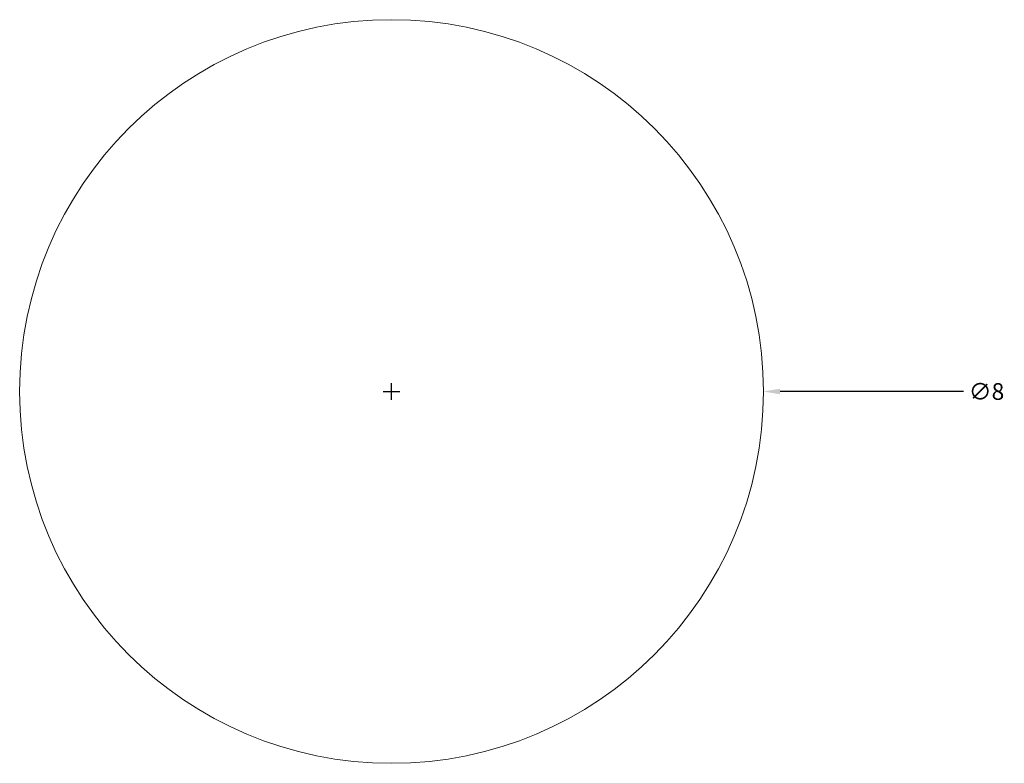
# Model space of a CAD drawing. Units: inches. Extents: x 369.5 to 380, y 21 to 29.
import ezdxf

# ---------------------------------------------------------------- set-up
doc = ezdxf.new("R2010")
doc.units = ezdxf.units.IN
doc.header["$MEASUREMENT"] = 0
doc.layers.add('M-CONS', color=7, linetype='Continuous', lineweight=18)
doc.layers.add('M-DIMS', color=2, linetype='Continuous', lineweight=18)
doc.styles.get("Standard").update_dxf_attribs({"font": 'arial.ttf'})
doc.dimstyles.get("Standard").update_dxf_attribs({"dimtxt": 0.18, "dimasz": 0.18, "dimexe": 0.18, "dimexo": 0.0625, "dimgap": 0.09, "dimtad": 0, "dimtih": 1, "dimtoh": 1, "dimdec": 4, "dimzin": 0, "dimdsep": 46, "dimtxsty": 'Standard', "dimcen": 0.09, "dimadec": 0, "dimazin": 0, "dimtfac": 1, "dimtdec": 4, "dimtofl": 0, "dimtmove": 0, "dimatfit": 3, "dimfxl": 1, "dimtolj": 1, "dimtzin": 0, "dimarcsym": 0})

# ---------------------------------------------------------------- blocks, each defined once
blk = doc.blocks.new('*D1')
at = {"layer": 'Defpoints', "color": 0, "transparency": 16777216}
for p in [(369.455, 25), (377.455, 25)]:
    blk.add_point(p, dxfattribs=at)
at = {"layer": 'M-DIMS', "color": 0, "lineweight": -2, "transparency": 16777216}
for p, q in [((373.365, 25), (373.545, 25)), ((373.455, 24.91), (373.455, 25.09)), ((379.608, 25), (377.635, 25))]:
    blk.add_line(p, q, dxfattribs=at)
at = {"layer": 'M-DIMS', "color": 0, "transparency": 16777216}
blk.add_solid([(377.635, 25.03), (377.635, 24.97), (377.455, 25)], dxfattribs=at)
at = {"layer": 'M-DIMS', "color": 0, "transparency": 16777216, "insert": (379.855, 25), "char_height": 0.18, "attachment_point": 5}
blk.add_mtext('\\A1;∅8', dxfattribs=at)

msp = doc.modelspace()

# ---------------------------------------------------------------- linework, layer by layer
at = {"layer": 'M-CONS'}
msp.add_circle((373.455, 25, 302.619), 4, dxfattribs=at)

# ---------------------------------------------------------------- dimensions: what is measured, and where the dimension line sits
at = {"layer": 'M-DIMS'}
dim = msp.add_diameter_dim_2p(p1=(369.455, 25), p2=(377.455, 25), dimstyle='Standard', override={"dimdec": 0, "dimlfac": 1, "dimrnd": 0, "dimzin": 0, "dimdsep": 46, "dimlunit": 2}, dxfattribs=at)
dim.commit()
dim.dimension.update_dxf_attribs({"geometry": '*D1', "text_midpoint": (379.855, 25), "dimtype": 163})

doc.saveas('drawing.dxf')
